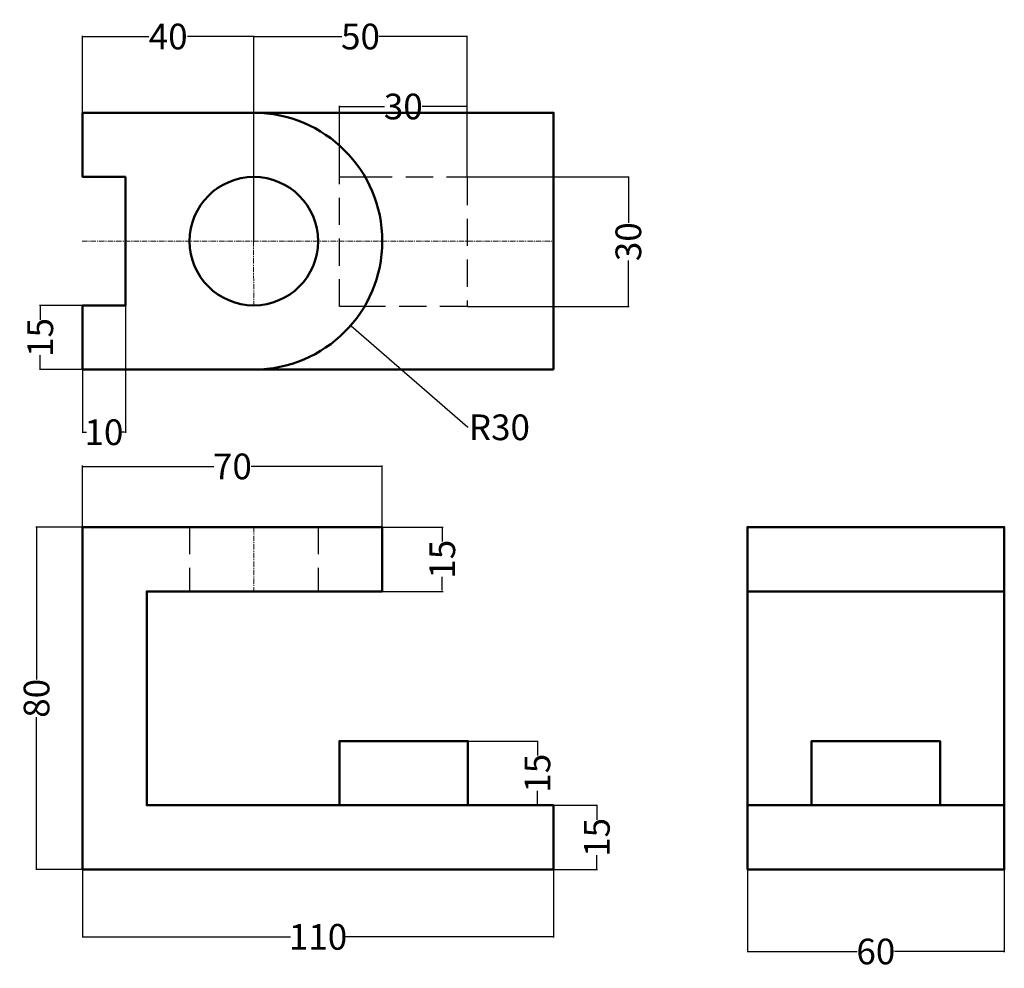
# Model space of a CAD drawing. Units: millimetres. Extents: x 12 to 242, y 10 to 232.
import ezdxf

# ---------------------------------------------------------------- set-up
doc = ezdxf.new("R2010")
doc.units = ezdxf.units.MM
doc.header["$MEASUREMENT"] = 0
doc.linetypes.add('CENTER', pattern=[2, 1.25, -0.25, 0.25, -0.25])
doc.linetypes.add('HIDDEN', pattern=[9.525, 6.35, -3.175])
for name, color, linetype, lineweight in [('M-CNTR', 1, 'CENTER', 18), ('M-DIMS', 2, 'Continuous', 25), ('M-HIDN', 4, 'HIDDEN', 25), ('M-OUTL', 7, 'Continuous', 50)]:
    doc.layers.add(name, color=color, linetype=linetype, lineweight=lineweight)
doc.styles.get("Standard").update_dxf_attribs({"font": 'arial.ttf'})
doc.dimstyles.get("Standard").update_dxf_attribs({"dimtxt": 6, "dimasz": 0.18, "dimexe": 0.18, "dimexo": 0.0625, "dimgap": 0.09, "dimtad": 0, "dimtoh": 1, "dimdec": 0, "dimzin": 0, "dimdsep": 46, "dimtxsty": 'Standard', "dimcen": 0.09, "dimadec": 0, "dimazin": 0, "dimtfac": 1, "dimtdec": 0, "dimtofl": 0, "dimtmove": 0, "dimatfit": 3, "dimfxl": 1, "dimtolj": 1, "dimtzin": 0, "dimarcsym": 0})

# ---------------------------------------------------------------- blocks, each defined once
blk = doc.blocks.new('*D1')
at = {"layer": 'Defpoints', "color": 0, "transparency": 16777216}
for p in [(26.76, 33.3), (136.76, 33.3), (136.76, 17.56)]:
    blk.add_point(p, dxfattribs=at)
at = {"layer": 'M-DIMS', "color": 0, "lineweight": -2, "transparency": 16777216}
for p, q in [((26.76, 33.24), (26.76, 17.38)), ((136.76, 33.24), (136.76, 17.38)), ((26.94, 17.56), (75.33, 17.56)), ((136.58, 17.56), (88.18, 17.56))]:
    blk.add_line(p, q, dxfattribs=at)
at = {"layer": 'M-DIMS', "color": 0, "transparency": 16777216}
for points in [[(26.94, 17.59), (26.94, 17.53), (26.76, 17.56)], [(136.58, 17.59), (136.58, 17.53), (136.76, 17.56)]]:
    blk.add_solid(points, dxfattribs=at)
at = {"layer": 'M-DIMS', "color": 0, "transparency": 16777216, "insert": (81.76, 17.56), "char_height": 6, "attachment_point": 5}
blk.add_mtext('\\A1;110', dxfattribs=at)
blk = doc.blocks.new('*D2')
at = {"layer": 'Defpoints', "color": 0, "transparency": 16777216}
for p in [(116.76, 63.3), (116.76, 48.3), (132.98, 48.3)]:
    blk.add_point(p, dxfattribs=at)
at = {"layer": 'M-DIMS', "color": 0, "lineweight": -2, "transparency": 16777216}
for p, q in [((116.82, 63.3), (133.16, 63.3)), ((132.98, 63.12), (132.98, 59.93)), ((132.98, 48.48), (132.98, 51.67)), ((116.82, 48.3), (133.16, 48.3))]:
    blk.add_line(p, q, dxfattribs=at)
at = {"layer": 'M-DIMS', "color": 0, "transparency": 16777216}
for points in [[(132.95, 63.12), (133.01, 63.12), (132.98, 63.3)], [(132.95, 48.48), (133.01, 48.48), (132.98, 48.3)]]:
    blk.add_solid(points, dxfattribs=at)
at = {"layer": 'M-DIMS', "color": 0, "transparency": 16777216, "insert": (132.98, 55.8), "char_height": 6, "attachment_point": 5, "rotation": 90}
blk.add_mtext('\\A1;15', dxfattribs=at)
blk = doc.blocks.new('*D3')
at = {"layer": 'Defpoints', "color": 0, "transparency": 16777216}
for p in [(136.76, 48.3), (136.76, 33.3), (146.87, 33.3)]:
    blk.add_point(p, dxfattribs=at)
at = {"layer": 'M-DIMS', "color": 0, "lineweight": -2, "transparency": 16777216}
for p, q in [((136.82, 48.3), (147.05, 48.3)), ((146.87, 48.12), (146.87, 44.93)), ((146.87, 33.48), (146.87, 36.67)), ((136.82, 33.3), (147.05, 33.3))]:
    blk.add_line(p, q, dxfattribs=at)
at = {"layer": 'M-DIMS', "color": 0, "transparency": 16777216}
for points in [[(146.84, 48.12), (146.9, 48.12), (146.87, 48.3)], [(146.84, 33.48), (146.9, 33.48), (146.87, 33.3)]]:
    blk.add_solid(points, dxfattribs=at)
at = {"layer": 'M-DIMS', "color": 0, "transparency": 16777216, "insert": (146.87, 40.8), "char_height": 6, "attachment_point": 5, "rotation": 90}
blk.add_mtext('\\A1;15', dxfattribs=at)
blk = doc.blocks.new('*D4')
at = {"layer": 'Defpoints', "color": 0, "transparency": 16777216}
for p in [(26.76, 113.3), (16.02, 33.3), (26.76, 33.3)]:
    blk.add_point(p, dxfattribs=at)
at = {"layer": 'M-DIMS', "color": 0, "lineweight": -2, "transparency": 16777216}
for p, q in [((26.7, 113.3), (15.84, 113.3)), ((16.02, 113.12), (16.02, 77.68)), ((16.02, 33.48), (16.02, 68.92)), ((26.7, 33.3), (15.84, 33.3))]:
    blk.add_line(p, q, dxfattribs=at)
at = {"layer": 'M-DIMS', "color": 0, "transparency": 16777216}
for points in [[(15.99, 113.12), (16.05, 113.12), (16.02, 113.3)], [(15.99, 33.48), (16.05, 33.48), (16.02, 33.3)]]:
    blk.add_solid(points, dxfattribs=at)
at = {"layer": 'M-DIMS', "color": 0, "transparency": 16777216, "insert": (16.02, 73.3), "char_height": 6, "attachment_point": 5, "rotation": 90}
blk.add_mtext('\\A1;80', dxfattribs=at)
blk = doc.blocks.new('*D5')
at = {"layer": 'Defpoints', "color": 0, "transparency": 16777216}
for p in [(96.76, 127.49), (26.76, 113.3), (96.76, 113.3)]:
    blk.add_point(p, dxfattribs=at)
at = {"layer": 'M-DIMS', "color": 0, "lineweight": -2, "transparency": 16777216}
for p, q in [((26.76, 113.36), (26.76, 127.67)), ((26.94, 127.49), (57.41, 127.49)), ((96.58, 127.49), (66.11, 127.49)), ((96.76, 113.36), (96.76, 127.67))]:
    blk.add_line(p, q, dxfattribs=at)
at = {"layer": 'M-DIMS', "color": 0, "transparency": 16777216}
for points in [[(26.94, 127.52), (26.94, 127.46), (26.76, 127.49)], [(96.58, 127.52), (96.58, 127.46), (96.76, 127.49)]]:
    blk.add_solid(points, dxfattribs=at)
at = {"layer": 'M-DIMS', "color": 0, "transparency": 16777216, "insert": (61.76, 127.49), "char_height": 6, "attachment_point": 5}
blk.add_mtext('\\A1;70', dxfattribs=at)
blk = doc.blocks.new('*D6')
at = {"layer": 'Defpoints', "color": 0, "transparency": 16777216}
for p in [(96.76, 113.3), (96.76, 98.3), (110.77, 98.3)]:
    blk.add_point(p, dxfattribs=at)
at = {"layer": 'M-DIMS', "color": 0, "lineweight": -2, "transparency": 16777216}
for p, q in [((96.82, 113.3), (110.95, 113.3)), ((110.77, 113.12), (110.77, 109.93)), ((110.77, 98.48), (110.77, 101.67)), ((96.82, 98.3), (110.95, 98.3))]:
    blk.add_line(p, q, dxfattribs=at)
at = {"layer": 'M-DIMS', "color": 0, "transparency": 16777216}
for points in [[(110.74, 113.12), (110.8, 113.12), (110.77, 113.3)], [(110.74, 98.48), (110.8, 98.48), (110.77, 98.3)]]:
    blk.add_solid(points, dxfattribs=at)
at = {"layer": 'M-DIMS', "color": 0, "transparency": 16777216, "insert": (110.77, 105.8), "char_height": 6, "attachment_point": 5, "rotation": 90}
blk.add_mtext('\\A1;15', dxfattribs=at)
blk = doc.blocks.new('*D7')
at = {"layer": 'Defpoints', "color": 0, "transparency": 16777216}
for p in [(182.01, 33.3), (242.01, 33.3), (242.01, 14.15)]:
    blk.add_point(p, dxfattribs=at)
at = {"layer": 'M-DIMS', "color": 0, "lineweight": -2, "transparency": 16777216}
for p, q in [((182.01, 33.24), (182.01, 13.97)), ((242.01, 33.24), (242.01, 13.97)), ((182.19, 14.15), (207.62, 14.15)), ((241.83, 14.15), (216.41, 14.15))]:
    blk.add_line(p, q, dxfattribs=at)
at = {"layer": 'M-DIMS', "color": 0, "transparency": 16777216}
for points in [[(182.19, 14.18), (182.19, 14.12), (182.01, 14.15)], [(241.83, 14.18), (241.83, 14.12), (242.01, 14.15)]]:
    blk.add_solid(points, dxfattribs=at)
at = {"layer": 'M-DIMS', "color": 0, "transparency": 16777216, "insert": (212.01, 14.15), "char_height": 6, "attachment_point": 5}
blk.add_mtext('\\A1;60', dxfattribs=at)
blk = doc.blocks.new('*D8')
at = {"layer": 'Defpoints', "color": 0, "transparency": 16777216}
for p in [(36.76, 165.12), (26.76, 150.12), (36.76, 135.48)]:
    blk.add_point(p, dxfattribs=at)
at = {"layer": 'M-DIMS', "color": 0, "lineweight": -2, "transparency": 16777216}
for p, q in [((36.76, 165.06), (36.76, 135.3)), ((26.76, 150.06), (26.76, 135.3)), ((26.94, 135.48), (27.66, 135.48)), ((36.58, 135.48), (35.85, 135.48))]:
    blk.add_line(p, q, dxfattribs=at)
at = {"layer": 'M-DIMS', "color": 0, "transparency": 16777216}
for points in [[(26.94, 135.51), (26.94, 135.45), (26.76, 135.48)], [(36.58, 135.51), (36.58, 135.45), (36.76, 135.48)]]:
    blk.add_solid(points, dxfattribs=at)
at = {"layer": 'M-DIMS', "color": 0, "transparency": 16777216, "insert": (31.76, 135.48), "char_height": 6, "attachment_point": 5}
blk.add_mtext('\\A1;10', dxfattribs=at)
blk = doc.blocks.new('*D9')
at = {"layer": 'Defpoints', "color": 0, "transparency": 16777216}
for p in [(26.76, 165.12), (16.89, 150.12), (26.76, 150.12)]:
    blk.add_point(p, dxfattribs=at)
at = {"layer": 'M-DIMS', "color": 0, "lineweight": -2, "transparency": 16777216}
for p, q in [((26.7, 165.12), (16.71, 165.12)), ((16.89, 164.94), (16.89, 161.75)), ((16.89, 150.3), (16.89, 153.49)), ((26.7, 150.12), (16.71, 150.12))]:
    blk.add_line(p, q, dxfattribs=at)
at = {"layer": 'M-DIMS', "color": 0, "transparency": 16777216}
for points in [[(16.86, 164.94), (16.92, 164.94), (16.89, 165.12)], [(16.86, 150.3), (16.92, 150.3), (16.89, 150.12)]]:
    blk.add_solid(points, dxfattribs=at)
at = {"layer": 'M-DIMS', "color": 0, "transparency": 16777216, "insert": (16.89, 157.62), "char_height": 6, "attachment_point": 5, "rotation": 90}
blk.add_mtext('\\A1;15', dxfattribs=at)
blk = doc.blocks.new('*D10')
at = {"layer": 'Defpoints', "color": 0, "transparency": 16777216}
for p in [(66.76, 227.94), (26.76, 210.12), (66.76, 180.12)]:
    blk.add_point(p, dxfattribs=at)
at = {"layer": 'M-DIMS', "color": 0, "lineweight": -2, "transparency": 16777216}
for p, q in [((26.76, 210.18), (26.76, 228.12)), ((26.94, 227.94), (42.26, 227.94)), ((66.58, 227.94), (51.26, 227.94)), ((66.76, 180.18), (66.76, 228.12))]:
    blk.add_line(p, q, dxfattribs=at)
at = {"layer": 'M-DIMS', "color": 0, "transparency": 16777216}
for points in [[(26.94, 227.97), (26.94, 227.91), (26.76, 227.94)], [(66.58, 227.97), (66.58, 227.91), (66.76, 227.94)]]:
    blk.add_solid(points, dxfattribs=at)
at = {"layer": 'M-DIMS', "color": 0, "transparency": 16777216, "insert": (46.76, 227.94), "char_height": 6, "attachment_point": 5}
blk.add_mtext('\\A1;40', dxfattribs=at)
blk = doc.blocks.new('*D11')
at = {"layer": 'Defpoints', "color": 0, "transparency": 16777216}
for p in [(116.58, 227.94), (66.76, 210.12), (116.58, 195)]:
    blk.add_point(p, dxfattribs=at)
at = {"layer": 'M-DIMS', "color": 0, "lineweight": -2, "transparency": 16777216}
for p, q in [((66.76, 210.18), (66.76, 228.12)), ((66.94, 227.94), (87.29, 227.94)), ((116.4, 227.94), (96.05, 227.94)), ((116.58, 195.06), (116.58, 228.12))]:
    blk.add_line(p, q, dxfattribs=at)
at = {"layer": 'M-DIMS', "color": 0, "transparency": 16777216}
for points in [[(66.94, 227.97), (66.94, 227.91), (66.76, 227.94)], [(116.4, 227.97), (116.4, 227.91), (116.58, 227.94)]]:
    blk.add_solid(points, dxfattribs=at)
at = {"layer": 'M-DIMS', "color": 0, "transparency": 16777216, "insert": (91.67, 227.94), "char_height": 6, "attachment_point": 5}
blk.add_mtext('\\A1;50', dxfattribs=at)
blk = doc.blocks.new('*D12')
at = {"layer": 'Defpoints', "color": 0, "transparency": 16777216}
for p in [(116.58, 211.59), (86.76, 195.12), (116.58, 195.12)]:
    blk.add_point(p, dxfattribs=at)
at = {"layer": 'M-DIMS', "color": 0, "lineweight": -2, "transparency": 16777216}
for p, q in [((86.76, 195.18), (86.76, 211.77)), ((86.94, 211.59), (97.29, 211.59)), ((116.4, 211.59), (106.04, 211.59)), ((116.58, 195.18), (116.58, 211.77))]:
    blk.add_line(p, q, dxfattribs=at)
at = {"layer": 'M-DIMS', "color": 0, "transparency": 16777216}
for points in [[(86.94, 211.62), (86.94, 211.56), (86.76, 211.59)], [(116.4, 211.62), (116.4, 211.56), (116.58, 211.59)]]:
    blk.add_solid(points, dxfattribs=at)
at = {"layer": 'M-DIMS', "color": 0, "transparency": 16777216, "insert": (101.67, 211.59), "char_height": 6, "attachment_point": 5}
blk.add_mtext('\\A1;30', dxfattribs=at)
blk = doc.blocks.new('*D13')
at = {"layer": 'Defpoints', "color": 0, "transparency": 16777216}
for p in [(66.76, 180.12), (89.38, 160.41)]:
    blk.add_point(p, dxfattribs=at)
at = {"layer": 'M-DIMS', "color": 0, "lineweight": -2, "transparency": 16777216}
for p, q in [((66.67, 180.12), (66.85, 180.12)), ((66.76, 180.03), (66.76, 180.21)), ((116.67, 136.63), (89.51, 160.29)), ((116.85, 136.63), (116.67, 136.63))]:
    blk.add_line(p, q, dxfattribs=at)
at = {"layer": 'M-DIMS', "color": 0, "transparency": 16777216}
blk.add_solid([(89.53, 160.32), (89.49, 160.27), (89.38, 160.41)], dxfattribs=at)
at = {"layer": 'M-DIMS', "color": 0, "transparency": 16777216, "insert": (124.1, 136.63), "char_height": 6, "attachment_point": 5}
blk.add_mtext('\\A1;R30', dxfattribs=at)
blk = doc.blocks.new('*D14')
at = {"layer": 'Defpoints', "color": 0, "transparency": 16777216}
for p in [(116.58, 195.12), (116.58, 164.87), (154.22, 164.87)]:
    blk.add_point(p, dxfattribs=at)
at = {"layer": 'M-DIMS', "color": 0, "lineweight": -2, "transparency": 16777216}
for p, q in [((116.64, 195.12), (154.4, 195.12)), ((154.22, 194.94), (154.22, 184.37)), ((154.22, 165.05), (154.22, 175.62)), ((116.64, 164.87), (154.4, 164.87))]:
    blk.add_line(p, q, dxfattribs=at)
at = {"layer": 'M-DIMS', "color": 0, "transparency": 16777216}
for points in [[(154.19, 194.94), (154.25, 194.94), (154.22, 195.12)], [(154.19, 165.05), (154.25, 165.05), (154.22, 164.87)]]:
    blk.add_solid(points, dxfattribs=at)
at = {"layer": 'M-DIMS', "color": 0, "transparency": 16777216, "insert": (154.22, 180), "char_height": 6, "attachment_point": 5, "rotation": 90}
blk.add_mtext('\\A1;30', dxfattribs=at)

msp = doc.modelspace()

# ---------------------------------------------------------------- linework, layer by layer
at = {"layer": 'M-CNTR'}
for p, q in [((26.64, 180.12), (136.88, 180.12)), ((66.67, 180.12), (66.76, 165.12)), ((66.76, 113.3), (66.76, 98.3))]:
    msp.add_line(p, q, dxfattribs=at)
at = {"layer": 'M-HIDN'}
for p, q in [((51.76, 113.3), (51.76, 98.3)), ((81.76, 113.3), (81.76, 98.3))]:
    msp.add_line(p, q, dxfattribs=at)
msp.add_lwpolyline([(116.58, 195.12), (116.58, 194.87), (116.58, 164.87), (92.59, 164.87), (86.76, 164.87), (86.76, 195.12), (92.74, 195.12)], close=True, dxfattribs=at)
at = {"layer": 'M-OUTL'}
for p, q in [((182.01, 98.3), (242.01, 98.3)), ((182.01, 48.3), (242.01, 48.3))]:
    msp.add_line(p, q, dxfattribs=at)
for points in [[(136.76, 150.12), (136.76, 210.12), (26.76, 210.12), (26.76, 195.12), (36.76, 195.12), (36.76, 165.12), (26.76, 165.12), (26.76, 150.12)], [(136.76, 33.3), (136.76, 48.3), (41.76, 48.3), (41.76, 98.3), (96.76, 98.3), (96.76, 113.3), (26.76, 113.3), (26.76, 33.3)], [(182.01, 33.3), (182.01, 113.3), (242.01, 113.3), (242.01, 33.3)]]:
    msp.add_lwpolyline(points, close=True, dxfattribs=at)
for points in [[(116.76, 48.3), (116.76, 63.3), (86.76, 63.3), (86.76, 48.3)], [(197.01, 48.3), (197.01, 63.3), (227.01, 63.3), (227.01, 48.3)]]:
    msp.add_lwpolyline(points, dxfattribs=at)
msp.add_circle((66.76, 180.12), 15, dxfattribs=at)
msp.add_arc((66.76, 180.12), 30, 270, 90, dxfattribs=at)

# ---------------------------------------------------------------- dimensions: what is measured, and where the dimension line sits
at = {"layer": 'M-DIMS'}
for base, p1, p2, picture, middle in [((66.76, 227.94), (26.76, 210.12), (66.76, 180.12), '*D10', (46.76, 227.94)), ((116.58, 227.94), (66.76, 210.12), (116.58, 195), '*D11', (91.67, 227.94)), ((116.58, 211.59), (86.76, 195.12), (116.58, 195.12), '*D12', (101.67, 211.59)), ((36.76, 135.48), (26.76, 150.12), (36.76, 165.12), '*D8', (31.76, 135.48)), ((96.76, 127.49), (26.76, 113.3), (96.76, 113.3), '*D5', (61.76, 127.49)), ((136.76, 17.56), (26.76, 33.3), (136.76, 33.3), '*D1', (81.76, 17.56)), ((242.01, 14.15), (182.01, 33.3), (242.01, 33.3), '*D7', (212.01, 14.15))]:
    dim = msp.add_linear_dim(base=base, p1=p1, p2=p2, dimstyle='Standard', override={"dimclrd": 0, "dimclre": 0, "dimclrt": 0}, dxfattribs=at)
    dim.commit()
    dim.dimension.update_dxf_attribs({"geometry": picture, "text_midpoint": middle})
for base, p1, p2, picture, middle in [((154.22, 164.87), (116.58, 195.12), (116.58, 164.87), '*D14', (154.22, 180)), ((16.89, 150.12), (26.76, 165.12), (26.76, 150.12), '*D9', (16.89, 157.62)), ((16.02, 33.3), (26.76, 113.3), (26.76, 33.3), '*D4', (16.02, 73.3)), ((110.77, 98.3), (96.76, 113.3), (96.76, 98.3), '*D6', (110.77, 105.8)), ((132.98, 48.3), (116.76, 63.3), (116.76, 48.3), '*D2', (132.98, 55.8)), ((146.87, 33.3), (136.76, 48.3), (136.76, 33.3), '*D3', (146.87, 40.8))]:
    dim = msp.add_linear_dim(base=base, p1=p1, p2=p2, angle=90, dimstyle='Standard', override={"dimclrd": 0, "dimclre": 0, "dimclrt": 0}, dxfattribs=at)
    dim.commit()
    dim.dimension.update_dxf_attribs({"geometry": picture, "text_midpoint": middle})
dim = msp.add_radius_dim(center=(66.76, 180.12), mpoint=(89.38, 160.41), dimstyle='Standard', override={"dimclrd": 0, "dimclre": 0, "dimclrt": 0}, dxfattribs=at)
dim.commit()
dim.dimension.update_dxf_attribs({"geometry": '*D13', "text_midpoint": (124.1, 136.63), "dimtype": 164})

doc.saveas('drawing.dxf')
